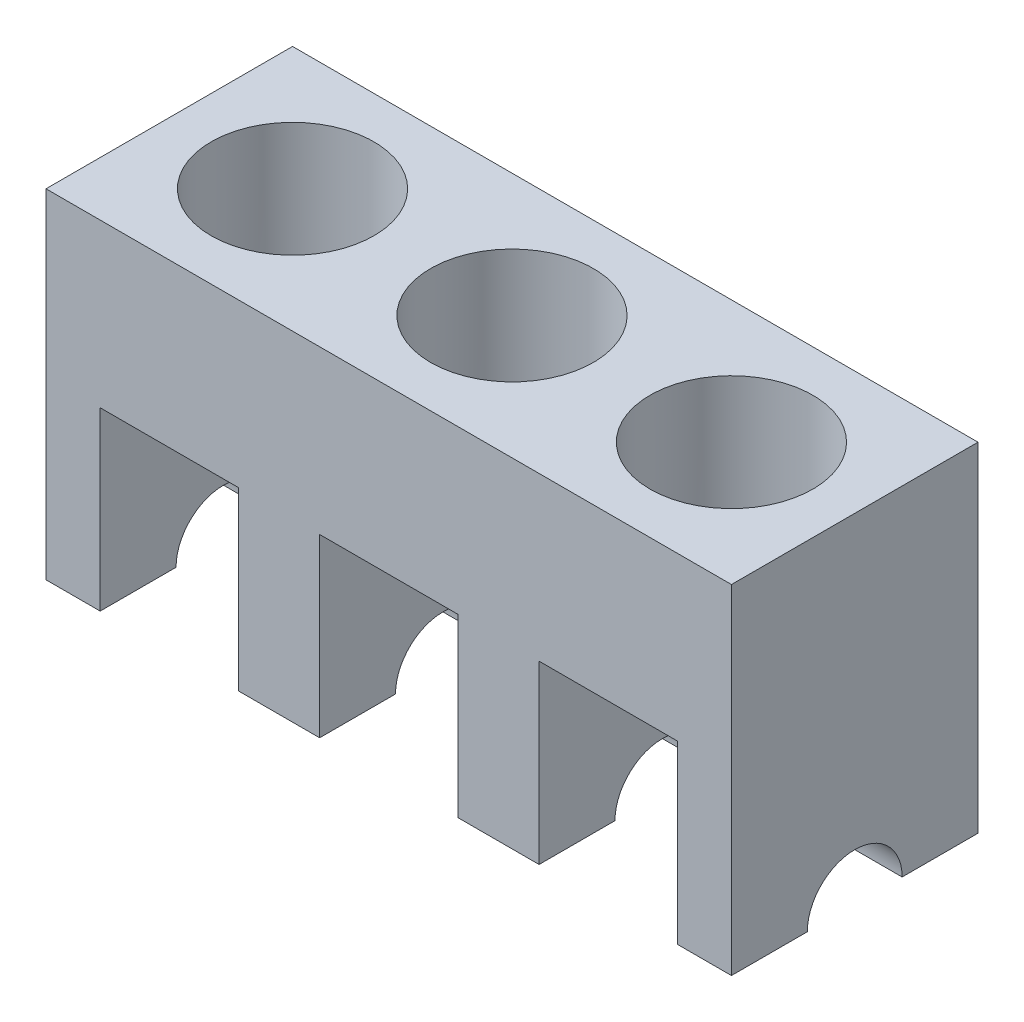
SolidWorks part; units mm, degrees
material "Plain Carbon Steel"
ref_plane "Front Plane" through (0, 0, 0) normal (0, 0, 1) x (1, 0, 0)
ref_plane "Top Plane" through (0, 0, 0) normal (0, 1, 0) x (1, 0, 0)
ref_plane "Right Plane" through (0, 0, 0) normal (1, 0, 0) x (0, 0, -1)
sketch "Block Profile Sketch" plane through (0, 0, 0) normal (0, 0, 1) x (1, 0, 0)
  line L0 (-106.5, -62.5) -> (-106.5, 2.5)
  line L1 (-126.5, -62.5) -> (-106.5, -62.5)
  line L2 (-126.5, -62.5) -> (-126.5, 62.5)
  line L3 (-126.5, 62.5) -> (126.5, 62.5)
  line L4 (126.5, -62.5) -> (126.5, 62.5)
  line L5 (-126.5, -62.5) -> (126.5, 62.5) construction
  line L6 (-126.5, 62.5) -> (55.5, -27.4209) construction
  line L7 (-106.5, 2.5) -> (-55.5, 2.5)
  line L8 (-55.5, 2.5) -> (-55.5, -62.5)
  line L9 (-25.5, -62.5) -> (-25.5, 2.5)
  line L10 (-25.5, 2.5) -> (25.5, 2.5)
  line L11 (25.5, 2.5) -> (25.5, -62.5)
  line L12 (55.5, -62.5) -> (55.5, 2.5)
  line L13 (55.5, 2.5) -> (106.5, 2.5)
  line L14 (106.5, 2.5) -> (106.5, -62.5)
  line L15 (-55.5, -62.5) -> (-25.5, -62.5)
  line L16 (25.5, -62.5) -> (55.5, -62.5)
  line L17 (106.5, -52.6186) -> (126.5, -62.5) construction
  line L18 (106.5, -62.5) -> (126.5, -62.5)
  point P0 (0, 0)
  dimension "D1" = 253
  dimension "D2" = 125
  dimension "D3" = 20
  dimension "D4" = 51
  dimension "D5" = 20
  dimension "D6" = 65
  dimension "D7" = 30
extrude "Block Body" add sketch "Block Profile Sketch" along normal mid plane 91
sketch "Crankshaft Bore Sketch" plane through (126.5, 0, 0) normal (1, 0, 0) x (0, 0, -1)
  line L0 (-45.5, -62.5) -> (45.5, -62.5) construction
  circle A0 centre (0, -62.5) radius 17.5
  dimension "D1" = 35
extrude "Crankshaft Bore Ø35" cut sketch "Crankshaft Bore Sketch" against normal through all
sketch "Cylinder Bores Sketch" plane through (0, 62.5, 0) normal (0, 1, 0) x (1, 0, 0)
  line L0 (-168.5525, 0) -> (170.4632, 0) construction
  line L1 (-126.5, -45.5) -> (-126.5, 45.5) construction
  line L2 (126.5, -45.5) -> (126.5, 45.5) construction
  circle A0 centre (-81, 0) radius 30.05
  circle A1 centre (0, 0) radius 30.05
  circle A2 centre (81, 0) radius 30.05
  dimension "D1" = 60.1
  dimension "D2" = 45.5
  dimension "D3" = 45.5
extrude "Cylinder Bores 3xØ45.5" cut sketch "Cylinder Bores Sketch" against normal blind 81
